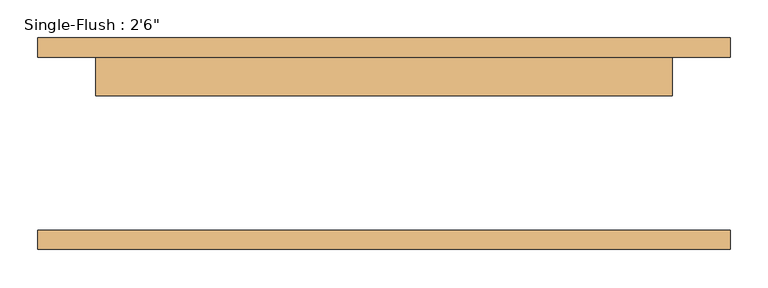
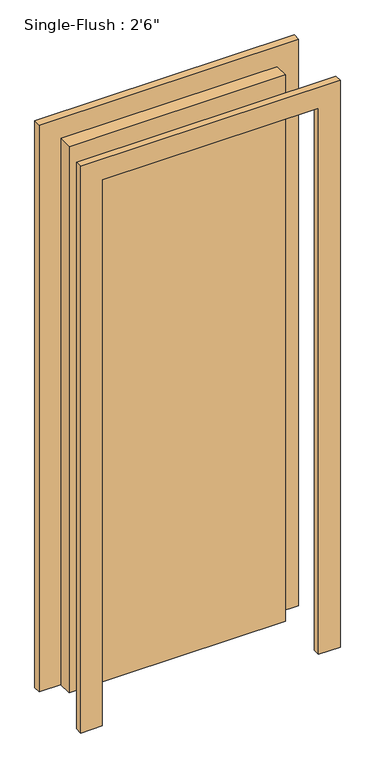
"""IFC4 building model written with IfcOpenShell, lengths in millimetres: door geometry."""

from ifc_helpers import new_model, si_unit, frame, origin, origin_with_axes, place, context, project, spatial, polyline, outline, extrude, source, transform, mapped, element, save


def door_a1484949(model_context):
    return source(origin(), model_context, "Body", "SweptSolid", [
        extrude(outline(polyline([(2108.2, -457.2), (0.0, -457.2), (0.0, -381.0), (2032.0, -381.0), (2032.0, 381.0), (0.0, 381.0), (0.0, 457.2), (2108.2, 457.2), (2108.2, -457.2)])), frame((0.0, 114.3, 0.0), z_axis=(0.0, 1.0, 0.0), x_axis=(0.0, 0.0, 1.0)), (0.0, 0.0, 1.0), 25.4),
        extrude(outline(polyline([(2108.2, 457.2), (2108.2, -457.2), (0.0, -457.2), (0.0, -381.0), (2032.0, -381.0), (2032.0, 381.0), (0.0, 381.0), (0.0, 457.2), (2108.2, 457.2)])), frame((0.0, -139.7, 0.0), z_axis=(0.0, 1.0, 0.0), x_axis=(0.0, 0.0, 1.0)), (0.0, 0.0, 1.0), 25.4),
        extrude(outline(polyline([(381.0, 63.5), (-381.0, 63.5), (-381.0, 114.3), (381.0, 114.3), (381.0, 63.5)])), origin_with_axes(), (0.0, 0.0, 1.0), 2032.0),
    ])


if __name__ == "__main__":
    model = new_model("IFC4")
    model_context = context("Model", 3, world=origin())
    ifc_project = project(units=[si_unit("LENGTHUNIT", "METRE", prefix="MILLI")], contexts=[model_context])
    site = spatial("IfcSite", under=ifc_project)
    building = spatial("IfcBuilding", under=site)
    placement = place(None, origin())
    door_shape = door_a1484949(model_context)
    element("IfcDoor", 1, ObjectType="Single-Flush : 2'6\"", at=placement, inside=building, context=model_context, shape_type="MappedRepresentation", body=[
        mapped(door_shape, transform((0.0, 0.0, 0.0), x_axis=(1.0, 0.0, 0.0), y_axis=(0.0, 1.0, 0.0), z_axis=(0.0, 0.0, 1.0))),
    ])
    save(model, "model.ifc")

# Revit data of these elements
# Type "Single-Flush : 2'6\""
#   Type Mark = "14"
#   Construction Type Id = "MDOOR"
#   Assembly Code = "C1020"
#   Analytic Construction = "Metal"
#   Rough Width = 2' - 6"
#   Rough Height = 7' - 0"
#   Thickness = 0' - 2"
#   Heat Transfer Coefficient (U) = 0.651978 BTU/(h·ft²·°F)
#   Height = 6' - 8"
#   Trim Projection Ext = 0' - 1"
#   Trim Projection Int = 0' - 1"
#   Trim Width = 0' - 3"
#   Width = 2' - 6"
#   Define Thermal Properties by = 1
#   Door Material = Door - Panel
#   Frame Material = Door - Frame
#   Visual Light Transmittance = 0
#   Solar Heat Gain Coefficient = 0
#   Function = (empty or 0)
#   Wall Closure = (empty or 0)
# Element 1 (IfcDoor, "Single-Flush : 2'6\"")
#   Materials on its faces: "Door - Frame", "Door - Panel"
# Materials
#   "Door - Panel": class "Wood", colour RGB 210 159 95, transparency 0, Cost = 0
#   "Door - Frame": colour RGB 118 70 51, transparency 0, Cost = 0
